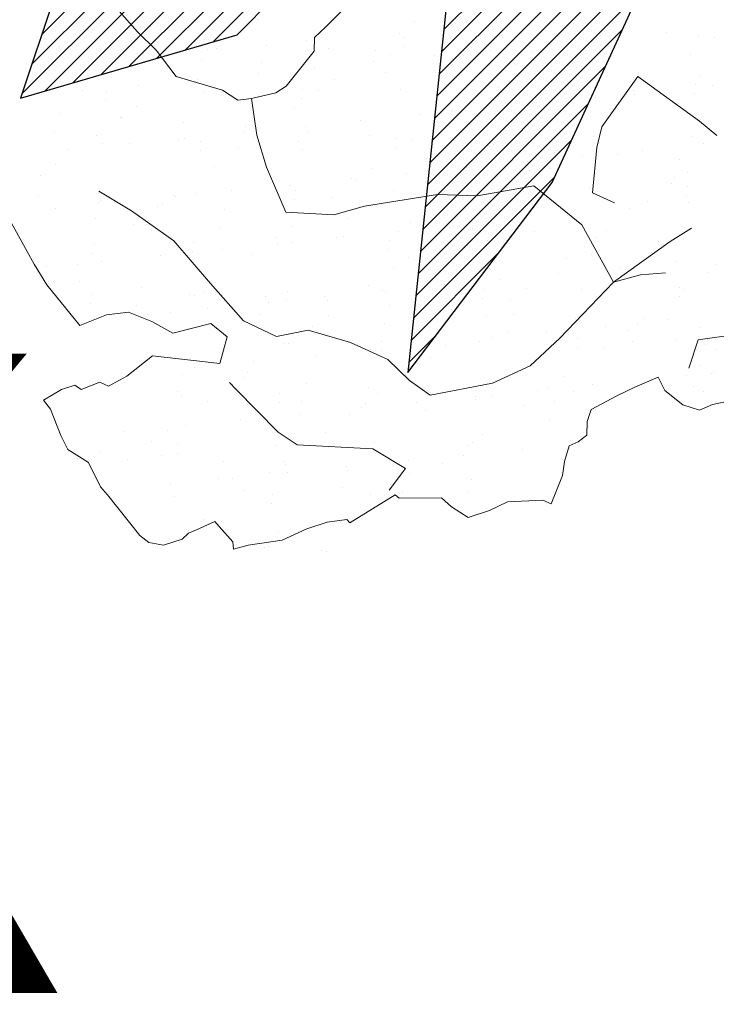
# Model space of a CAD drawing. Units: inches. Extents: x 1986 to 21484, y -1816 to 2016.
# Tile 51 of 85: x 3656.5 to 3664.13, y 1860.02 to 1870.8. Entities that reach past the tile are written whole.
import ezdxf

# ---------------------------------------------------------------- set-up
doc = ezdxf.new("R2010")
doc.units = ezdxf.units.IN
for name, color, linetype, lineweight in [('A-ANNO-TEXT', 7, 'Continuous', 18), ('L-PLNT', 84, 'Continuous', 13), ('vfolhas', 114, 'Continuous', 5)]:
    doc.layers.add(name, color=color, linetype=linetype, lineweight=lineweight)
doc.layers.add('vfolha2', color=110, linetype='Continuous')
doc.layers.add('vfolhas2', color=102, linetype='Continuous')
doc.styles.get("Standard").update_dxf_attribs({"font": 'arial.ttf'})
pattern_1 = [(45, (-2446.5133113, 50.986076), (-0.004419417382, 0.004419417382), [])]

# ---------------------------------------------------------------- blocks, each defined once
blk = doc.blocks.new('arbusto_PB_verde_grande')
at = {"layer": 'vfolha2'}
h = blk.add_hatch(dxfattribs=at)
h.set_pattern_fill('ANSI31', color=256, scale=0.05, style=0)
h.set_pattern_definition(pattern_1)
h.paths.add_polyline_path([(0.02944, 0.35651), (0.00028, 0.09048), (0.02625, -0.03934), (0.047, 0.06233), (0.06189, 0.09731), (0.09372, 0.26573), (0.09955, 0.43473), (0.08789, 0.61313), (0.0645, 0.72266), (0.04988, 0.6851), (0.0236, 0.51294)])
h.paths.add_polyline_path([(0.30106, 0.43789), (0.14225, 0.24871), (0.26685, 0.30022)])
h.paths.add_polyline_path([(0.37995, 0.22817), (0.23697, 0.15193), (0.18428, 0.09364), (0.11122, 0.04358), (0.02625, -0.03934), (0.28061, 0.04667), (0.36829, 0.07798), (0.46756, 0.11239), (0.61068, 0.19376), (0.71585, 0.27823), (0.55813, 0.25948)])
h.paths.add_polyline_path([(0.56101, -0.29441), (0.72752, -0.32573), (0.59024, -0.2412), (0.42962, -0.15982), (0.02625, -0.03934), (0.14922, -0.14107), (0.18838, -0.16604), (0.41501, -0.24435)])
h.paths.add_polyline_path([(-0.27429, -0.44776), (-0.30352, -0.72628), (-0.23923, -0.64175), (-0.15457, -0.45716), (0.02625, -0.03934), (-0.16328, -0.25376)])
h.paths.add_polyline_path([(-0.51963, -0.24744), (-0.67736, -0.32573), (-0.59558, -0.35072), (-0.40574, -0.32882), (-0.21007, -0.20995), (0.02625, -0.03934), (-0.14874, -0.06595), (-0.31518, -0.09101), (-0.41452, -0.15048)])
h.paths.add_polyline_path([(-0.52546, 0.25007), (-0.70947, 0.24698), (-0.51963, 0.1093), (-0.32979, 0.02167), (-0.07567, -0.0128), (-0.04234, -0.02148), (-0.35024, 0.1312)])
at = {"layer": 'vfolhas'}
h = blk.add_hatch(dxfattribs=at)
h.set_pattern_fill('ANSI31', color=256, scale=0.05, style=0)
h.set_pattern_definition(pattern_1)
h.paths.add_polyline_path([(-0.57219, 0.06233), (-0.7153, 0.10298), (-0.67736, 0.08107), (-0.62769, 0.01536), (-0.56347, -0.04095), (-0.26461, -0.0834), (-0.14874, -0.06595), (-0.10151, -0.05877), (-0.20418, -0.0472), (-0.40279, -0.00339)])
h.paths.add_polyline_path([(-0.56347, -0.04095), (-0.58279, -0.02401), (-0.72992, -0.09726), (-0.4334, -0.1679), (-0.41452, -0.15048), (-0.31518, -0.09101), (-0.26461, -0.0834)])
h.paths.add_polyline_path([(-0.2769, -0.47267), (-0.27429, -0.44776), (-0.16328, -0.25376), (0.02625, -0.03934), (-0.21007, -0.20995), (-0.2672, -0.24466), (-0.36485, -0.35697), (-0.42907, -0.46341), (-0.47586, -0.60425), (-0.37946, -0.57603)])
at = {"layer": 'vfolha2'}
for p, q in [((-0.27429, -0.44776), (-0.30352, -0.72628)), ((-0.30352, -0.72628), (-0.23923, -0.64175))]:
    blk.add_line(p, q, dxfattribs=at)
at = {"layer": 'vfolhas2'}
for p, q in [((-0.23923, -0.64175), (-0.15457, -0.45716)), ((-0.42907, -0.46341), (-0.47586, -0.60425)), ((-0.37946, -0.57603), (-0.2769, -0.47267)), ((-0.47586, -0.60425), (-0.37946, -0.57603))]:
    blk.add_line(p, q, dxfattribs=at)
blk = doc.blocks.new('PLANT-SHRUB')
for p, q in [((2179.266, 1899.378), (2179.436, 1899.277)), ((2179.436, 1899.277), (2179.582, 1899.222)), ((2179.582, 1899.222), (2179.674, 1899.057)), ((2179.407, 1899.104), (2179.407, 1899.104)), ((2178.578, 1898.995), (2179.065, 1898.651)), ((2179.19, 1899.031), (2179.19, 1899.031)), ((2179.208, 1899.017), (2179.208, 1899.017)), ((2179.451, 1898.985), (2179.451, 1898.985)), ((2179.674, 1899.057), (2179.711, 1898.806)), ((2179.005, 1898.857), (2179.005, 1898.857)), ((2179.065, 1898.651), (2179.352, 1898.808)), ((2179.236, 1898.871), (2179.236, 1898.871)), ((2179.292, 1898.839), (2179.292, 1898.839)), ((2179.424, 1898.851), (2179.424, 1898.851)), ((2179.711, 1898.806), (2179.665, 1898.65)), ((2181.164, 1898.718), (2181.466, 1898.859)), ((2181.466, 1898.859), (2181.507, 1898.768)), ((2181.466, 1898.859), (2181.466, 1898.859)), ((2181.507, 1898.768), (2181.8, 1898.516)), ((2178.993, 1898.717), (2178.993, 1898.717)), ((2179.043, 1898.738), (2179.043, 1898.738)), ((2179.124, 1898.685), (2179.124, 1898.685)), ((2179.153, 1898.712), (2179.153, 1898.712)), ((2181.045, 1898.621), (2181.164, 1898.718)), ((2181.164, 1898.718), (2181.164, 1898.718)), ((2178.963, 1898.568), (2178.963, 1898.568)), ((2179.065, 1898.651), (2179.065, 1898.651)), ((2179.665, 1898.65), (2179.926, 1898.554)), ((2179.729, 1898.617), (2179.729, 1898.617)), ((2179.926, 1898.554), (2180.136, 1898.49)), ((2180.564, 1898.47), (2180.669, 1898.58)), ((2180.669, 1898.58), (2180.788, 1898.567)), ((2180.788, 1898.567), (2180.889, 1898.53)), ((2180.889, 1898.53), (2181.045, 1898.621)), ((2180.912, 1898.562), (2180.912, 1898.562)), ((2179.239, 1898.48), (2179.239, 1898.48)), ((2180.136, 1898.49), (2180.44, 1898.406)), ((2180.136, 1898.49), (2180.136, 1898.49)), ((2180.44, 1898.406), (2180.564, 1898.47)), ((2180.839, 1898.494), (2180.839, 1898.494)), ((2181.8, 1898.516), (2182.011, 1898.452)), ((2182.011, 1898.452), (2182.235, 1898.347)), ((2182.235, 1898.347), (2182.286, 1898.137)), ((2179.165, 1898.261), (2179.165, 1898.261)), ((2178.357, 1898.181), (2178.357, 1898.181)), ((2178.477, 1898.192), (2178.477, 1898.192)), ((2178.801, 1898.149), (2178.801, 1898.149)), ((2178.892, 1898.162), (2178.892, 1898.162)), ((2179.601, 1898.179), (2179.601, 1898.179)), ((2180.244, 1898.222), (2180.244, 1898.222)), ((2180.441, 1898.13), (2180.441, 1898.13)), ((2180.846, 1898.177), (2180.846, 1898.177)), ((2181.291, 1898.208), (2181.291, 1898.208)), ((2182.04, 1898.143), (2182.04, 1898.143)), ((2182.286, 1898.137), (2182.299, 1897.99)), ((2178.818, 1898.094), (2178.818, 1898.094)), ((2179.344, 1898.078), (2179.344, 1898.078)), ((2179.433, 1898.072), (2179.433, 1898.072)), ((2179.552, 1898.05), (2179.552, 1898.05)), ((2180.677, 1898.069), (2180.677, 1898.069)), ((2181.922, 1898.067), (2181.922, 1898.067)), ((2179.877, 1898.008), (2179.877, 1898.008)), ((2180.42, 1897.936), (2180.42, 1897.936)), ((2180.628, 1897.909), (2180.628, 1897.909)), ((2182.299, 1897.99), (2182.638, 1897.674)), ((2178.658, 1897.86), (2178.658, 1897.86)), ((2178.823, 1897.873), (2179.038, 1897.701)), ((2179.704, 1897.847), (2179.704, 1897.847)), ((2180.093, 1897.811), (2180.093, 1897.811)), ((2180.726, 1897.852), (2180.726, 1897.852)), ((2180.953, 1897.866), (2180.953, 1897.866)), ((2181.806, 1897.813), (2181.806, 1897.813)), ((2178.282, 1897.712), (2178.554, 1897.658)), ((2178.42, 1897.73), (2178.42, 1897.73)), ((2179.038, 1897.701), (2179.311, 1897.558)), ((2180.019, 1897.744), (2180.019, 1897.744)), ((2181.496, 1897.795), (2181.496, 1897.795)), ((2181.642, 1897.779), (2181.642, 1897.779)), ((2181.704, 1897.767), (2181.704, 1897.767)), ((2182.029, 1897.724), (2182.029, 1897.724)), ((2178.554, 1897.658), (2179.311, 1897.558)), ((2179.311, 1897.558), (2180.157, 1897.601)), ((2180.157, 1897.601), (2180.601, 1897.601)), ((2180.157, 1897.601), (2180.157, 1897.601)), ((2180.601, 1897.601), (2181.032, 1897.458)), ((2182.572, 1897.653), (2182.572, 1897.653)), ((2182.638, 1897.674), (2182.647, 1897.62)), ((2182.647, 1897.62), (2183.217, 1897.503)), ((2178.117, 1897.486), (2178.117, 1897.486)), ((2178.641, 1897.567), (2178.641, 1897.567)), ((2179.311, 1897.558), (2179.134, 1896.861)), ((2179.14, 1897.491), (2179.14, 1897.491)), ((2179.885, 1897.565), (2179.885, 1897.565)), ((2181.13, 1897.562), (2181.13, 1897.562)), ((2182.365, 1897.486), (2182.661, 1897.536)), ((2182.365, 1897.486), (2182.365, 1897.486)), ((2182.48, 1897.085), (2182.365, 1897.486)), ((2182.374, 1897.56), (2182.374, 1897.56)), ((2183.217, 1897.503), (2183.217, 1897.453)), ((2183.619, 1897.558), (2183.619, 1897.558)), ((2183.648, 1897.511), (2183.648, 1897.511)), ((2178.072, 1897.411), (2178.072, 1897.411)), ((2179.622, 1897.379), (2179.622, 1897.379)), ((2180.219, 1897.452), (2180.219, 1897.452)), ((2181.032, 1897.458), (2181.62, 1897.085)), ((2181.221, 1897.393), (2181.221, 1897.393)), ((2181.265, 1897.438), (2181.265, 1897.438)), ((2181.294, 1897.46), (2181.294, 1897.46)), ((2182.288, 1897.443), (2182.288, 1897.443)), ((2182.844, 1897.428), (2182.844, 1897.428)), ((2183.217, 1897.453), (2183.395, 1897.325)), ((2183.367, 1897.404), (2183.367, 1897.404)), ((2177.999, 1897.344), (2177.999, 1897.344)), ((2183.395, 1897.325), (2183.606, 1897.229)), ((2177.387, 1897.16), (2177.416, 1896.917)), ((2177.9, 1897.233), (2177.9, 1897.233)), ((2178.034, 1897.18), (2178.034, 1897.18)), ((2178.108, 1897.206), (2178.108, 1897.206)), ((2178.433, 1897.163), (2178.433, 1897.163)), ((2179.278, 1897.178), (2179.278, 1897.178)), ((2180.523, 1897.176), (2180.523, 1897.176)), ((2181.768, 1897.174), (2181.768, 1897.174)), ((2183.012, 1897.171), (2183.012, 1897.171)), ((2183.606, 1897.229), (2183.89, 1897.133)), ((2177.553, 1897.129), (2177.553, 1897.129)), ((2177.865, 1897.073), (2177.865, 1897.073)), ((2178.633, 1897.09), (2178.633, 1897.09)), ((2178.976, 1897.091), (2178.976, 1897.091)), ((2179.11, 1897.071), (2179.11, 1897.071)), ((2179.184, 1897.064), (2179.184, 1897.064)), ((2179.274, 1897.06), (2179.274, 1897.06)), ((2179.679, 1897.077), (2179.679, 1897.077)), ((2180.355, 1897.068), (2180.355, 1897.068)), ((2180.701, 1897.082), (2180.701, 1897.082)), ((2181.599, 1897.066), (2181.599, 1897.066)), ((2181.62, 1897.085), (2181.677, 1896.813)), ((2181.781, 1897.043), (2181.781, 1897.043)), ((2182.48, 1897.085), (2182.48, 1897.085)), ((2183.054, 1896.483), (2182.48, 1897.085)), ((2182.496, 1897.109), (2182.496, 1897.109)), ((2182.844, 1897.064), (2182.844, 1897.064)), ((2183.89, 1897.133), (2184.197, 1896.918)), ((2184.045, 1897.077), (2184.045, 1897.077)), ((2184.088, 1897.062), (2184.088, 1897.062)), ((2177.601, 1896.979), (2177.601, 1896.979)), ((2179.2, 1896.993), (2179.2, 1896.993)), ((2179.509, 1897.021), (2179.509, 1897.021)), ((2180.052, 1896.95), (2180.052, 1896.95)), ((2180.823, 1897.028), (2180.823, 1897.028)), ((2182.422, 1897.042), (2182.422, 1897.042)), ((2182.827, 1897.03), (2182.827, 1897.03)), ((2183.849, 1897.035), (2183.849, 1897.035)), ((2177.416, 1896.917), (2177.574, 1896.1)), ((2178.807, 1896.687), (2178.707, 1896.931)), ((2179.134, 1896.861), (2179.225, 1896.191)), ((2180.26, 1896.922), (2180.26, 1896.922)), ((2180.585, 1896.88), (2180.585, 1896.88)), ((2184.197, 1896.918), (2184.343, 1896.84)), ((2184.343, 1896.84), (2184.293, 1896.776)), ((2177.046, 1896.729), (2177.046, 1896.729)), ((2179.115, 1896.72), (2179.115, 1896.72)), ((2181.127, 1896.808), (2181.127, 1896.808)), ((2181.335, 1896.781), (2181.335, 1896.781)), ((2181.66, 1896.738), (2181.66, 1896.738)), ((2181.677, 1896.813), (2181.691, 1896.483)), ((2183.697, 1896.759), (2183.697, 1896.759)), ((2184.293, 1896.776), (2184.288, 1896.552)), ((2177.253, 1896.661), (2177.253, 1896.661)), ((2178.092, 1896.716), (2178.092, 1896.716)), ((2178.434, 1896.358), (2178.807, 1896.687)), ((2178.802, 1896.628), (2178.802, 1896.628)), ((2178.807, 1896.687), (2178.807, 1896.687)), ((2180.194, 1896.682), (2180.194, 1896.682)), ((2180.402, 1896.642), (2180.402, 1896.642)), ((2180.475, 1896.71), (2180.475, 1896.71)), ((2181.24, 1896.668), (2181.24, 1896.668)), ((2182.024, 1896.677), (2182.024, 1896.677)), ((2182.203, 1896.667), (2182.203, 1896.667)), ((2182.263, 1896.673), (2182.263, 1896.673)), ((2182.411, 1896.639), (2182.411, 1896.639)), ((2183.342, 1896.634), (2183.342, 1896.634)), ((2183.624, 1896.691), (2183.624, 1896.691)), ((2177.073, 1896.568), (2177.073, 1896.568)), ((2177.18, 1896.593), (2177.18, 1896.593)), ((2178.318, 1896.566), (2178.318, 1896.566)), ((2179.562, 1896.564), (2179.562, 1896.564)), ((2180.807, 1896.562), (2180.807, 1896.562)), ((2182.052, 1896.559), (2182.052, 1896.559)), ((2182.736, 1896.596), (2182.736, 1896.596)), ((2183.279, 1896.525), (2183.279, 1896.525)), ((2183.296, 1896.557), (2183.296, 1896.557)), ((2184.288, 1896.552), (2184.288, 1896.479)), ((2181.691, 1896.483), (2181.863, 1896.067)), ((2183.111, 1896.239), (2183.054, 1896.483)), ((2183.487, 1896.498), (2183.487, 1896.498)), ((2183.812, 1896.455), (2183.812, 1896.455)), ((2184.288, 1896.479), (2184.495, 1896.407)), ((2184.495, 1896.407), (2184.582, 1896.375)), ((2176.664, 1896.361), (2176.664, 1896.361)), ((2176.989, 1896.318), (2176.989, 1896.318)), ((2177.528, 1896.359), (2177.528, 1896.359)), ((2178.239, 1896.228), (2178.434, 1896.358)), ((2178.455, 1896.31), (2178.455, 1896.31)), ((2178.608, 1896.32), (2178.608, 1896.32)), ((2179.654, 1896.307), (2179.654, 1896.307)), ((2180.676, 1896.312), (2180.676, 1896.312)), ((2181.603, 1896.291), (2181.603, 1896.291)), ((2181.677, 1896.359), (2181.677, 1896.359)), ((2183.226, 1896.327), (2183.226, 1896.327)), ((2184.355, 1896.383), (2184.355, 1896.383)), ((2184.563, 1896.356), (2184.563, 1896.356)), ((2184.582, 1896.375), (2184.678, 1896.375)), ((2184.678, 1896.375), (2184.875, 1896.284)), ((2176.782, 1896.228), (2176.782, 1896.228)), ((2177.531, 1896.247), (2177.531, 1896.247)), ((2177.574, 1896.1), (2178.239, 1896.228)), ((2177.74, 1896.219), (2177.74, 1896.219)), ((2178.381, 1896.242), (2178.381, 1896.242)), ((2179.225, 1896.191), (2179.751, 1895.847)), ((2180.004, 1896.278), (2180.004, 1896.278)), ((2181.756, 1896.273), (2181.756, 1896.273)), ((2182.802, 1896.26), (2182.802, 1896.26)), ((2183.126, 1895.58), (2183.111, 1896.239)), ((2183.824, 1896.264), (2183.824, 1896.264)), ((2184.875, 1896.284), (2184.971, 1896.151)), ((2177.711, 1896.18), (2177.711, 1896.18)), ((2178.064, 1896.177), (2178.064, 1896.177)), ((2178.607, 1896.105), (2178.607, 1896.105)), ((2178.815, 1896.078), (2178.815, 1896.078)), ((2178.956, 1896.177), (2178.956, 1896.177)), ((2180.2, 1896.175), (2180.2, 1896.175)), ((2181.445, 1896.173), (2181.445, 1896.173)), ((2182.69, 1896.17), (2182.69, 1896.17)), ((2183.934, 1896.168), (2183.934, 1896.168)), ((2184.971, 1896.151), (2184.99, 1896.028)), ((2177.542, 1896.072), (2177.542, 1896.072)), ((2178.787, 1896.07), (2178.787, 1896.07)), ((2179.14, 1896.035), (2179.14, 1896.035)), ((2180.032, 1896.068), (2180.032, 1896.068)), ((2181.276, 1896.065), (2181.276, 1896.065)), ((2181.863, 1896.067), (2182.107, 1895.652)), ((2182.521, 1896.063), (2182.521, 1896.063)), ((2182.878, 1896.008), (2182.878, 1896.008)), ((2183.766, 1896.061), (2183.766, 1896.061)), ((2184.427, 1895.976), (2184.427, 1895.976)), ((2184.99, 1896.028), (2184.944, 1895.46)), ((2177.021, 1895.959), (2177.021, 1895.959)), ((2177.983, 1895.878), (2177.983, 1895.878)), ((2178.067, 1895.945), (2178.067, 1895.945)), ((2179.089, 1895.95), (2179.089, 1895.95)), ((2179.582, 1895.891), (2179.582, 1895.891)), ((2179.656, 1895.959), (2179.656, 1895.959)), ((2179.683, 1895.964), (2179.683, 1895.964)), ((2179.891, 1895.936), (2179.891, 1895.936)), ((2180.169, 1895.912), (2180.169, 1895.912)), ((2180.216, 1895.893), (2180.216, 1895.893)), ((2181.205, 1895.927), (2181.205, 1895.927)), ((2181.215, 1895.898), (2181.215, 1895.898)), ((2182.238, 1895.903), (2182.238, 1895.903)), ((2182.805, 1895.941), (2182.805, 1895.941)), ((2183.317, 1895.864), (2183.317, 1895.864)), ((2179.751, 1895.847), (2180.059, 1895.539)), ((2180.759, 1895.822), (2180.759, 1895.822)), ((2180.967, 1895.795), (2180.967, 1895.795)), ((2181.292, 1895.752), (2181.292, 1895.752)), ((2184.363, 1895.851), (2184.363, 1895.851)), ((2181.835, 1895.68), (2181.835, 1895.68)), ((2182.043, 1895.653), (2182.043, 1895.653)), ((2182.107, 1895.652), (2182.408, 1895.466)), ((2184.08, 1895.657), (2184.08, 1895.657)), ((2177.503, 1895.589), (2177.503, 1895.589)), ((2177.635, 1895.559), (2177.635, 1895.559)), ((2177.995, 1895.565), (2177.995, 1895.565)), ((2178.582, 1895.55), (2178.582, 1895.55)), ((2179.24, 1895.563), (2179.24, 1895.563)), ((2179.629, 1895.537), (2179.629, 1895.537)), ((2180.059, 1895.539), (2180.729, 1895.086)), ((2180.484, 1895.561), (2180.484, 1895.561)), ((2180.651, 1895.542), (2180.651, 1895.542)), ((2180.784, 1895.541), (2180.784, 1895.541)), ((2180.858, 1895.608), (2180.858, 1895.608)), ((2181.729, 1895.558), (2181.729, 1895.558)), ((2182.368, 1895.61), (2182.368, 1895.61)), ((2182.407, 1895.576), (2182.407, 1895.576)), ((2182.911, 1895.539), (2182.911, 1895.539)), ((2182.974, 1895.556), (2182.974, 1895.556)), ((2183.126, 1895.48), (2183.126, 1895.58)), ((2184.006, 1895.59), (2184.006, 1895.59)), ((2184.218, 1895.554), (2184.218, 1895.554)), ((2177.562, 1895.492), (2177.562, 1895.492)), ((2179.185, 1895.527), (2179.185, 1895.527)), ((2181.73, 1895.503), (2181.73, 1895.503)), ((2182.408, 1895.466), (2182.552, 1895.093)), ((2182.777, 1895.489), (2182.777, 1895.489)), ((2183.119, 1895.511), (2183.119, 1895.511)), ((2183.444, 1895.468), (2183.444, 1895.468)), ((2183.799, 1895.494), (2183.799, 1895.494)), ((2184.878, 1895.455), (2184.878, 1895.455)), ((2184.944, 1895.46), (2184.939, 1895.346)), ((2183.986, 1895.397), (2183.986, 1895.397)), ((2184.194, 1895.37), (2184.194, 1895.37)), ((2184.519, 1895.327), (2184.519, 1895.327)), ((2184.939, 1895.346), (2184.852, 1895.062)), ((2182.059, 1895.257), (2182.059, 1895.257)), ((2183.063, 1895.254), (2182.803, 1895.098)), ((2183.063, 1895.254), (2183.063, 1895.254)), ((2183.543, 1894.689), (2183.063, 1895.254)), ((2183.608, 1895.225), (2183.608, 1895.225)), ((2177.696, 1895.19), (2177.696, 1895.19)), ((2178.042, 1895.175), (2178.042, 1895.175)), ((2178.239, 1895.119), (2178.239, 1895.119)), ((2178.633, 1895.176), (2178.633, 1895.176)), ((2178.763, 1895.141), (2178.763, 1895.141)), ((2178.837, 1895.208), (2178.837, 1895.208)), ((2179.064, 1895.18), (2179.064, 1895.18)), ((2179.878, 1895.174), (2179.878, 1895.174)), ((2180.144, 1895.141), (2180.144, 1895.141)), ((2180.386, 1895.176), (2180.386, 1895.176)), ((2181.122, 1895.172), (2181.122, 1895.172)), ((2181.19, 1895.128), (2181.19, 1895.128)), ((2181.985, 1895.19), (2181.985, 1895.19)), ((2182.212, 1895.133), (2182.212, 1895.133)), ((2182.367, 1895.17), (2182.367, 1895.17)), ((2183.611, 1895.167), (2183.611, 1895.167)), ((2178.447, 1895.092), (2178.447, 1895.092)), ((2178.464, 1895.069), (2178.464, 1895.069)), ((2178.772, 1895.049), (2178.772, 1895.049)), ((2179.709, 1895.067), (2179.709, 1895.067)), ((2180.729, 1895.086), (2181.037, 1894.923)), ((2180.954, 1895.065), (2180.954, 1895.065)), ((2182.198, 1895.062), (2182.198, 1895.062)), ((2182.552, 1895.093), (2182.537, 1894.548)), ((2182.803, 1895.098), (2182.834, 1894.869)), ((2183.292, 1895.094), (2183.292, 1895.094)), ((2183.443, 1895.06), (2183.443, 1895.06)), ((2184.338, 1895.081), (2184.338, 1895.081)), ((2184.687, 1895.058), (2184.687, 1895.058)), ((2184.852, 1895.062), (2184.921, 1894.804)), ((2179.315, 1894.977), (2179.315, 1894.977)), ((2179.523, 1894.95), (2179.523, 1894.95)), ((2179.848, 1894.907), (2179.848, 1894.907)), ((2181.037, 1894.923), (2181.4, 1894.543)), ((2178.557, 1894.78), (2178.557, 1894.78)), ((2179.965, 1894.79), (2179.965, 1894.79)), ((2180.038, 1894.858), (2180.038, 1894.858)), ((2180.39, 1894.836), (2180.39, 1894.836)), ((2180.598, 1894.808), (2180.598, 1894.808)), ((2181.588, 1894.825), (2181.588, 1894.825)), ((2182.834, 1894.869), (2183.209, 1894.661)), ((2184.921, 1894.804), (2184.871, 1894.639)), ((2178.365, 1894.776), (2178.365, 1894.776)), ((2179.603, 1894.767), (2179.603, 1894.767)), ((2180.626, 1894.772), (2180.626, 1894.772)), ((2180.923, 1894.765), (2180.923, 1894.765)), ((2181.466, 1894.694), (2181.466, 1894.694)), ((2181.705, 1894.733), (2181.705, 1894.733)), ((2182.751, 1894.719), (2182.751, 1894.719)), ((2183.543, 1894.689), (2183.543, 1894.689)), ((2183.9, 1894.662), (2183.543, 1894.689)), ((2183.774, 1894.724), (2183.774, 1894.724)), ((2181.674, 1894.667), (2181.674, 1894.667)), ((2181.999, 1894.624), (2181.999, 1894.624)), ((2183.209, 1894.661), (2183.292, 1894.412)), ((2184.12, 1894.602), (2183.9, 1894.662)), ((2184.161, 1894.506), (2184.12, 1894.602)), ((2184.871, 1894.639), (2184.757, 1894.351)), ((2178.917, 1894.562), (2178.917, 1894.562)), ((2180.161, 1894.56), (2180.161, 1894.56)), ((2181.4, 1894.543), (2181.219, 1894.036)), ((2181.24, 1894.507), (2181.24, 1894.507)), ((2181.406, 1894.558), (2181.406, 1894.558)), ((2182.537, 1894.548), (2182.509, 1893.932)), ((2182.542, 1894.552), (2182.542, 1894.552)), ((2182.651, 1894.555), (2182.651, 1894.555)), ((2182.75, 1894.525), (2182.75, 1894.525)), ((2182.789, 1894.475), (2182.789, 1894.475)), ((2183.075, 1894.482), (2183.075, 1894.482)), ((2184.367, 1894.424), (2184.161, 1894.506)), ((2179.039, 1894.41), (2179.039, 1894.41)), ((2179.567, 1894.426), (2179.567, 1894.426)), ((2180.119, 1894.371), (2180.119, 1894.371)), ((2181.165, 1894.358), (2181.165, 1894.358)), ((2181.166, 1894.439), (2181.166, 1894.439)), ((2182.187, 1894.363), (2182.187, 1894.363)), ((2183.292, 1894.412), (2183.406, 1894.162)), ((2184.381, 1894.342), (2184.367, 1894.424)), ((2184.757, 1894.351), (2184.747, 1894.227)), ((2183.267, 1894.324), (2183.267, 1894.324)), ((2184.523, 1894.277), (2184.381, 1894.342)), ((2184.747, 1894.227), (2184.523, 1894.277)), ((2179.555, 1894.173), (2179.555, 1894.173)), ((2180.799, 1894.171), (2180.799, 1894.171)), ((2182.044, 1894.169), (2182.044, 1894.169)), ((2182.441, 1894.156), (2182.441, 1894.156)), ((2183.289, 1894.167), (2183.289, 1894.167)), ((2183.406, 1894.162), (2183.604, 1894.017)), ((2184.747, 1894.227), (2184.747, 1894.227)), ((2179.146, 1894.039), (2179.146, 1894.039)), ((2179.219, 1894.107), (2179.219, 1894.107)), ((2179.386, 1894.066), (2179.386, 1894.066)), ((2180.631, 1894.064), (2180.631, 1894.064)), ((2180.768, 1894.075), (2180.768, 1894.075)), ((2181.219, 1894.036), (2181.056, 1893.71)), ((2181.875, 1894.061), (2181.875, 1894.061)), ((2182.368, 1894.088), (2182.368, 1894.088)), ((2183.12, 1894.059), (2183.12, 1894.059)), ((2178.946, 1893.991), (2178.946, 1893.991)), ((2179.154, 1893.964), (2179.154, 1893.964)), ((2179.479, 1893.921), (2179.479, 1893.921)), ((2179.578, 1893.997), (2179.578, 1893.997)), ((2180.601, 1894.001), (2180.601, 1894.001)), ((2181.68, 1893.963), (2181.68, 1893.963)), ((2182.509, 1893.932), (2182.624, 1893.373)), ((2182.726, 1893.949), (2182.726, 1893.949)), ((2183.604, 1894.017), (2183.895, 1893.902)), ((2183.749, 1893.954), (2183.749, 1893.954)), ((2180.022, 1893.849), (2180.022, 1893.849)), ((2180.23, 1893.822), (2180.23, 1893.822)), ((2183.895, 1893.902), (2183.854, 1893.331)), ((2180.421, 1893.756), (2180.421, 1893.756)), ((2180.555, 1893.779), (2180.555, 1893.779)), ((2181.056, 1893.71), (2180.822, 1893.378)), ((2181.098, 1893.708), (2181.098, 1893.708)), ((2181.97, 1893.724), (2181.97, 1893.724)), ((2183.569, 1893.738), (2183.569, 1893.738)), ((2183.643, 1893.805), (2183.643, 1893.805)), ((2180.093, 1893.601), (2180.093, 1893.601)), ((2180.347, 1893.689), (2180.347, 1893.689)), ((2181.306, 1893.68), (2181.306, 1893.68)), ((2181.631, 1893.638), (2181.631, 1893.638)), ((2179.839, 1893.559), (2179.839, 1893.559)), ((2180.456, 1893.539), (2179.969, 1893.468)), ((2180.588, 1893.513), (2180.456, 1893.539)), ((2180.822, 1893.378), (2180.588, 1893.513)), ((2181.083, 1893.557), (2181.083, 1893.557)), ((2181.14, 1893.588), (2181.14, 1893.588)), ((2182.162, 1893.593), (2182.162, 1893.593)), ((2182.174, 1893.566), (2182.174, 1893.566)), ((2182.328, 1893.555), (2182.328, 1893.555)), ((2182.382, 1893.539), (2182.382, 1893.539)), ((2182.707, 1893.496), (2182.707, 1893.496)), ((2183.241, 1893.554), (2183.241, 1893.554)), ((2183.573, 1893.552), (2183.573, 1893.552)), ((2179.969, 1893.468), (2179.863, 1893.362)), ((2180.822, 1893.378), (2180.822, 1893.378)), ((2180.822, 1893.378), (2180.948, 1893.289)), ((2181.622, 1893.405), (2181.622, 1893.405)), ((2183.249, 1893.424), (2183.249, 1893.424)), ((2183.457, 1893.397), (2183.457, 1893.397)), ((2179.695, 1893.362), (2179.368, 1893.353)), ((2179.695, 1893.362), (2179.695, 1893.362)), ((2179.863, 1893.362), (2179.695, 1893.362)), ((2179.863, 1893.362), (2179.863, 1893.362)), ((2179.949, 1893.324), (2179.949, 1893.324)), ((2180.948, 1893.289), (2180.993, 1893.092)), ((2181.548, 1893.338), (2181.548, 1893.338)), ((2182.624, 1893.373), (2182.738, 1892.972)), ((2183.171, 1893.373), (2183.171, 1893.373)), ((2183.782, 1893.354), (2183.782, 1893.354)), ((2183.854, 1893.331), (2183.802, 1893.071)), ((2180.477, 1893.17), (2180.477, 1893.17)), ((2180.575, 1893.231), (2180.575, 1893.231)), ((2181.655, 1893.193), (2181.655, 1893.193)), ((2181.721, 1893.168), (2181.721, 1893.168)), ((2182.701, 1893.179), (2182.701, 1893.179)), ((2182.966, 1893.166), (2182.966, 1893.166)), ((2183.723, 1893.184), (2183.723, 1893.184)), ((2180.308, 1893.063), (2180.308, 1893.063)), ((2180.993, 1893.092), (2181.261, 1892.636)), ((2181.553, 1893.061), (2181.553, 1893.061)), ((2182.797, 1893.058), (2182.797, 1893.058)), ((2183.802, 1893.071), (2183.646, 1892.457)), ((2181.151, 1892.973), (2181.151, 1892.973)), ((2182.75, 1892.987), (2182.75, 1892.987)), ((2182.824, 1893.055), (2182.824, 1893.055)), ((2180.186, 1892.793), (2180.186, 1892.793)), ((2181.114, 1892.818), (2181.114, 1892.818)), ((2182.137, 1892.823), (2182.137, 1892.823)), ((2183.216, 1892.784), (2183.216, 1892.784)), ((2180.729, 1892.721), (2180.729, 1892.721)), ((2180.803, 1892.655), (2180.803, 1892.655)), ((2180.937, 1892.694), (2180.937, 1892.694)), ((2181.261, 1892.636), (2181.225, 1892.278)), ((2181.262, 1892.651), (2181.262, 1892.651)), ((2180.729, 1892.587), (2180.729, 1892.587)), ((2180.761, 1892.556), (2180.761, 1892.556)), ((2181.805, 1892.58), (2181.805, 1892.58)), ((2182.005, 1892.554), (2182.005, 1892.554)), ((2182.013, 1892.552), (2182.013, 1892.552)), ((2182.352, 1892.623), (2182.352, 1892.623)), ((2183.25, 1892.551), (2183.25, 1892.551)), ((2180.55, 1892.461), (2180.55, 1892.461)), ((2181.63, 1892.422), (2181.63, 1892.422)), ((2182.338, 1892.51), (2182.338, 1892.51)), ((2182.676, 1892.409), (2182.676, 1892.409)), ((2182.881, 1892.438), (2182.881, 1892.438)), ((2183.089, 1892.411), (2183.089, 1892.411)), ((2182.004, 1892.304), (2182.004, 1892.304)), ((2181.225, 1892.278), (2181.234, 1891.991)), ((2181.931, 1892.236), (2181.931, 1892.236)), ((2181.398, 1892.167), (2181.398, 1892.167)), ((2182.643, 1892.165), (2182.643, 1892.165)), ((2181.089, 1892.048), (2181.089, 1892.048)), ((2181.234, 1891.991), (2181.225, 1891.643)), ((2181.23, 1892.06), (2181.23, 1892.06)), ((2182.112, 1892.053), (2182.112, 1892.053)), ((2182.475, 1892.058), (2182.475, 1892.058)), ((2181.533, 1891.872), (2181.533, 1891.872)), ((2181.604, 1891.652), (2181.604, 1891.652)), ((2181.645, 1891.566), (2181.645, 1891.566)), ((2181.682, 1891.553), (2181.682, 1891.553)), ((2182.651, 1891.639), (2182.651, 1891.639)), ((2181.97, 1891.523), (2181.97, 1891.523)), ((2182.086, 1891.282), (2182.086, 1891.282))]:
    blk.add_line(p, q)

msp = doc.modelspace()

# ---------------------------------------------------------------- block references
at = {"layer": 'L-PLNT', "rotation": 223.1883365522388}
msp.add_blockref('PLANT-SHRUB', (3953.27, 4742.965), dxfattribs=at)
at = {"layer": 'L-PLNT', "xscale": 24.60366729364114, "yscale": 24.60366729364114, "zscale": 24.60366729364114}
msp.add_blockref('arbusto_PB_verde_grande', (3668.218, 1884.805), dxfattribs=at)

# ---------------------------------------------------------------- texts
at = {"layer": 'A-ANNO-TEXT', "insert": (3605.478, 1867.143), "char_height": 7, "attachment_point": 1}
msp.add_mtext_dynamic_manual_height_columns("{\\fTimes New Roman|b0|i0|c0|p18;4' SETBACK}", width=105.61268, gutter_width=12.5, heights=[0], dxfattribs=at)

doc.saveas('drawing.dxf')
